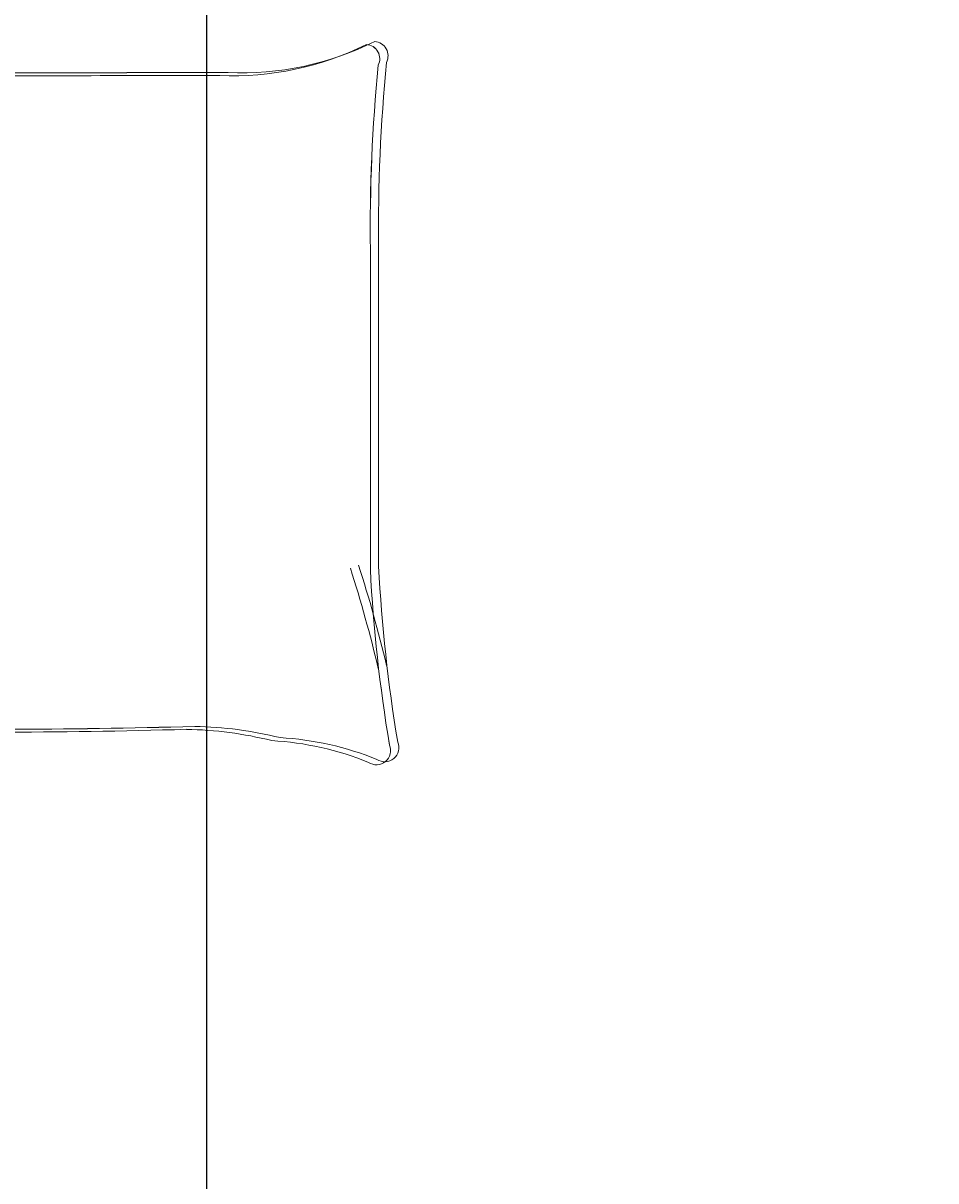
# Model space of a CAD drawing. Units: inches. Extents: x 1601 to 2297, y 1496 to 2631.
# Tile 42 of 57: x 1750 to 1820, y 2391 to 2480. Entities that reach past the tile are written whole.
import ezdxf

# ---------------------------------------------------------------- set-up
doc = ezdxf.new("R2010")
doc.units = ezdxf.units.IN
doc.layers.add('A-ANNO-DIMS', color=2, linetype='Continuous', lineweight=18)
doc.layers.add('A-FURN', color=8, linetype='Continuous', lineweight=18)
doc.styles.get("Standard").update_dxf_attribs({"font": 'arial.ttf'})
doc.dimstyles.get("Standard").update_dxf_attribs({"dimtxt": 0.18, "dimasz": 0.18, "dimexe": 0.18, "dimexo": 0.0625, "dimgap": 0.09, "dimtad": 0, "dimtih": 1, "dimtoh": 1, "dimdec": 4, "dimzin": 0, "dimdsep": 46, "dimtxsty": 'Standard', "dimcen": 0.09, "dimadec": 0, "dimazin": 0, "dimtfac": 1, "dimtdec": 4, "dimtofl": 0, "dimtmove": 0, "dimatfit": 3, "dimfxl": 1, "dimtolj": 1, "dimtzin": 0, "dimarcsym": 0})

# ---------------------------------------------------------------- blocks, each defined once
blk = doc.blocks.new('BED-DOUBLE')
for p, q in [((27.746, 52.867), (24.495, 49.162)), ((27.746, 52.867), (24.495, 49.162)), ((27.746, 52.867), (24.495, 49.162)), ((27.746, 52.867), (24.495, 49.162)), ((28.385, 53.096), (25.135, 49.39)), ((28.385, 53.096), (25.135, 49.39)), ((28.385, 53.096), (25.135, 49.39)), ((28.385, 53.096), (25.135, 49.39)), ((29.49, 52.947), (27.746, 52.867, 3.871)), ((29.49, 52.947), (27.746, 52.867, 3.871)), ((29.49, 52.947), (27.746, 52.867, 3.871)), ((29.49, 52.947), (27.746, 52.867, 3.871)), ((28.365, 51.33), (27.746, 52.867)), ((28.365, 51.33), (27.746, 52.867)), ((28.365, 51.33), (27.746, 52.867)), ((28.365, 51.33), (27.746, 52.867)), ((30.13, 53.175), (28.385, 53.096, 3.871)), ((30.13, 53.175), (28.385, 53.096, 3.871)), ((30.13, 53.175), (28.385, 53.096, 3.871)), ((30.13, 53.175), (28.385, 53.096, 3.871)), ((29.004, 51.559), (28.385, 53.096)), ((29.004, 51.558), (28.385, 53.096)), ((29.004, 51.559), (28.385, 53.096)), ((29.004, 51.558), (28.385, 53.096)), ((0, 51.494), (0.639, 51.493)), ((0, 3.475), (0, 51.494)), ((0, 51.494), (0.639, 51.493)), ((0, 3.475), (0, 51.494)), ((0, 51.265), (26.61, 51.265)), ((0, 51.265), (26.61, 51.265)), ((0, 51.265), (26.61, 51.265)), ((0, 51.265), (26.61, 51.265)), ((0.639, 51.494), (27.249, 51.494)), ((0.639, 51.494), (27.249, 51.494)), ((0.639, 51.493), (27.249, 51.493)), ((0.639, 51.493), (27.249, 51.493)), ((1.533, 3.475), (1.533, 51.265)), ((1.533, 3.475), (1.533, 51.265)), ((1.533, 3.475), (1.533, 51.265)), ((1.533, 3.475), (1.533, 51.265)), ((2.173, 3.703), (2.173, 51.494)), ((2.173, 3.703), (2.173, 51.494)), ((2.173, 3.703), (2.173, 51.493)), ((2.173, 3.703), (2.173, 51.493)), ((17.212, 50.926), (14.073, 50.151)), ((17.212, 50.926), (14.073, 50.151)), ((17.212, 50.926), (14.073, 50.151)), ((17.212, 50.926), (14.073, 50.151)), ((16.808, 45.795), (17.212, 50.926)), ((16.808, 45.794), (17.212, 50.926)), ((16.808, 45.795), (17.212, 50.926)), ((16.808, 45.794), (17.212, 50.926)), ((28.055, 48.233), (28.365, 51.33)), ((28.055, 48.233), (28.365, 51.33)), ((28.055, 48.233), (28.365, 51.33)), ((28.055, 48.233), (28.365, 51.33)), ((28.695, 48.461), (29.004, 51.559)), ((28.695, 48.461), (29.004, 51.559)), ((28.695, 48.461), (29.004, 51.558)), ((28.695, 48.461), (29.004, 51.558)), ((2.557, 50.112), (2.46, 44.709)), ((2.557, 50.112), (2.46, 44.709)), ((2.557, 50.111), (2.46, 44.709)), ((2.557, 50.111), (2.46, 44.709)), ((2.557, 50.112), (5.768, 49.733)), ((2.557, 50.112), (5.768, 49.733)), ((2.557, 50.111), (5.768, 49.733)), ((2.557, 50.111), (5.768, 49.733)), ((3.196, 50.34), (3.099, 44.938)), ((3.196, 50.34), (3.099, 44.938)), ((3.196, 50.34), (3.099, 44.938)), ((3.196, 50.34), (3.099, 44.938)), ((3.196, 50.34), (6.407, 49.961)), ((3.196, 50.34), (6.407, 49.961)), ((3.196, 50.34), (6.407, 49.961)), ((3.196, 50.34), (6.407, 49.961)), ((5.768, 49.733), (8.338, 50.328)), ((5.768, 49.733), (8.338, 50.328)), ((5.768, 49.733), (8.338, 50.328)), ((5.768, 49.733), (8.338, 50.328)), ((6.407, 49.961), (8.977, 50.557)), ((6.407, 49.961), (8.977, 50.557)), ((6.407, 49.961), (8.977, 50.556)), ((6.407, 49.961), (8.977, 50.556)), ((11.829, 50.112), (8.257, 49.309)), ((11.829, 50.112), (8.257, 49.309)), ((11.829, 50.112), (8.257, 49.309)), ((11.829, 50.112), (8.257, 49.309)), ((8.338, 50.328), (9.384, 49.814)), ((8.338, 50.328), (9.384, 49.814)), ((8.338, 50.328), (9.384, 49.814)), ((8.338, 50.328), (9.384, 49.814)), ((12.468, 50.34), (8.896, 49.538)), ((12.468, 50.34), (8.896, 49.537)), ((12.468, 50.34), (8.896, 49.538)), ((12.468, 50.34), (8.896, 49.537)), ((8.977, 50.557), (10.024, 50.043)), ((8.977, 50.557), (10.024, 50.043)), ((8.977, 50.556), (10.024, 50.042)), ((8.977, 50.556), (10.024, 50.042)), ((13.434, 49.923), (11.829, 50.112)), ((13.434, 49.922), (11.829, 50.112)), ((13.434, 49.923), (11.829, 50.112)), ((13.434, 49.922), (11.829, 50.112)), ((14.073, 50.151), (12.468, 50.34)), ((14.073, 50.151), (12.468, 50.34)), ((14.073, 50.151), (12.468, 50.34)), ((14.073, 50.151), (12.468, 50.34)), ((16.573, 50.698), (13.434, 49.923)), ((16.573, 50.698), (13.434, 49.922)), ((16.573, 50.698), (13.434, 49.923)), ((16.573, 50.698), (13.434, 49.922)), ((16.169, 45.566), (16.573, 50.698)), ((16.169, 45.566), (16.573, 50.698)), ((16.169, 45.566), (16.573, 50.698)), ((16.169, 45.566), (16.573, 50.698)), ((8.257, 49.309), (5.578, 48.128)), ((8.257, 49.309), (5.578, 48.128)), ((8.257, 49.309), (5.578, 48.128)), ((8.257, 49.309), (5.578, 48.128)), ((8.896, 49.538), (6.218, 48.356)), ((8.896, 49.538), (6.218, 48.356)), ((8.896, 49.537), (6.218, 48.356)), ((8.896, 49.537), (6.218, 48.356)), ((24.495, 49.162), (22.329, 46.219)), ((24.495, 49.162), (22.329, 46.219)), ((24.495, 49.162), (22.329, 46.219)), ((24.495, 49.162), (22.329, 46.219)), ((25.135, 49.39), (22.968, 46.448)), ((25.135, 49.39), (22.968, 46.448)), ((25.135, 49.39), (22.968, 46.448)), ((25.135, 49.39), (22.968, 46.448)), ((28.365, 44.361), (28.055, 48.233)), ((28.365, 44.361), (28.055, 48.233)), ((28.365, 44.361), (28.055, 48.233)), ((28.365, 44.361), (28.055, 48.233)), ((29.004, 44.589), (28.695, 48.461)), ((29.004, 44.589), (28.695, 48.461)), ((29.004, 44.589), (28.695, 48.461)), ((29.004, 44.589), (28.695, 48.461)), ((22.968, 46.448), (20.956, 40.872)), ((22.968, 46.448), (20.956, 40.872)), ((22.968, 46.448), (20.956, 40.872)), ((22.968, 46.448), (20.956, 40.872)), ((2.46, 44.709), (2.542, 45.712)), ((2.46, 44.709), (2.542, 45.712)), ((2.46, 44.709), (2.542, 45.712)), ((2.46, 44.709), (2.542, 45.712)), ((2.542, 45.712), (3.069, 41.914)), ((2.542, 45.712), (3.069, 41.914)), ((2.542, 45.712), (3.069, 41.914)), ((2.542, 45.712), (3.069, 41.914)), ((3.099, 44.938), (3.181, 45.941)), ((3.099, 44.938), (3.181, 45.941)), ((3.099, 44.938), (3.181, 45.94)), ((3.099, 44.938), (3.181, 45.94)), ((3.181, 45.941), (3.709, 42.143)), ((3.181, 45.941), (3.709, 42.143)), ((3.181, 45.94), (3.709, 42.142)), ((3.181, 45.94), (3.709, 42.142)), ((16.726, 43.606), (16.169, 45.566)), ((16.726, 43.606), (16.169, 45.566)), ((16.726, 43.606), (16.169, 45.566)), ((16.726, 43.606), (16.169, 45.566)), ((17.365, 43.834), (16.808, 45.795)), ((17.365, 43.834), (16.808, 45.795)), ((17.365, 43.834), (16.808, 45.794)), ((17.365, 43.834), (16.808, 45.794)), ((22.329, 46.219), (20.316, 40.644)), ((22.329, 46.219), (20.316, 40.644)), ((22.329, 46.219), (20.317, 40.644)), ((22.329, 46.219), (20.317, 40.644)), ((16.934, 36.824), (17.365, 43.834)), ((16.934, 36.824), (17.365, 43.834)), ((16.934, 36.824), (17.365, 43.834)), ((16.934, 36.824), (17.365, 43.834)), ((28.829, 40.954), (28.365, 44.361)), ((28.829, 40.953), (28.365, 44.361)), ((28.829, 40.954), (28.365, 44.361)), ((28.829, 40.953), (28.365, 44.361)), ((29.468, 41.182), (29.004, 44.589)), ((29.469, 41.182), (29.004, 44.589)), ((29.468, 41.182), (29.004, 44.589)), ((29.469, 41.182), (29.004, 44.589)), ((16.295, 36.596), (16.726, 43.606)), ((16.295, 36.596), (16.726, 43.606)), ((16.295, 36.596), (16.726, 43.606)), ((16.295, 36.596), (16.726, 43.606)), ((3.709, 42.143), (5.061, 36.723)), ((3.709, 42.143), (5.061, 36.723)), ((3.709, 42.142), (5.061, 36.723)), ((3.709, 42.142), (5.061, 36.723)), ((3.069, 41.914), (4.422, 36.495)), ((3.069, 41.914), (4.422, 36.495)), ((3.069, 41.914), (4.422, 36.495)), ((3.069, 41.914), (4.422, 36.495)), ((30.397, 39.169), (29.468, 41.182)), ((30.397, 39.169), (29.468, 41.182)), ((30.397, 39.168), (29.469, 41.182)), ((30.397, 39.168), (29.469, 41.182)), ((20.316, 40.644), (17.383, 32.306)), ((20.317, 40.644), (17.383, 32.306)), ((20.316, 40.644), (17.383, 32.306)), ((20.317, 40.644), (17.383, 32.306)), ((20.956, 40.872), (18.022, 32.534)), ((20.956, 40.872), (18.022, 32.534)), ((20.956, 40.872), (18.022, 32.534)), ((20.956, 40.872), (18.022, 32.534)), ((29.758, 38.94), (28.829, 40.954)), ((29.758, 38.94), (28.829, 40.954)), ((29.758, 38.94), (28.829, 40.953)), ((29.758, 38.94), (28.829, 40.953)), ((4.313, 39.428), (3.717, 37.363)), ((4.313, 39.428), (3.717, 37.363)), ((4.313, 39.428), (3.718, 37.363)), ((4.313, 39.428), (3.718, 37.363)), ((79.245, 15.063), (79.245, 39.677)), ((79.245, 15.063), (79.245, 39.677)), ((79.245, 15.063), (79.245, 39.677)), ((79.245, 15.063), (79.245, 39.677)), ((79.884, 15.292), (79.884, 39.905)), ((79.884, 15.291), (79.884, 39.905)), ((79.884, 15.292), (79.884, 39.905)), ((79.884, 15.291), (79.884, 39.905)), ((3.673, 39.2), (3.078, 37.135)), ((3.673, 39.2), (3.078, 37.135)), ((3.673, 39.2), (3.078, 37.135)), ((3.673, 39.2), (3.078, 37.135)), ((30.377, 36.462), (29.758, 38.94)), ((30.377, 36.462), (29.758, 38.94)), ((30.377, 36.462), (29.758, 38.94)), ((30.377, 36.462), (29.758, 38.94)), ((31.016, 36.691), (30.397, 39.169)), ((31.016, 36.691), (30.397, 39.169)), ((31.016, 36.691), (30.397, 39.168)), ((31.016, 36.691), (30.397, 39.168)), ((3.078, 37.135), (2.537, 34.204)), ((3.078, 37.135), (2.537, 34.204)), ((3.078, 37.135), (2.537, 34.204)), ((3.078, 37.135), (2.537, 34.204)), ((3.717, 37.363), (3.176, 34.433)), ((3.718, 37.363), (3.176, 34.433)), ((3.717, 37.363), (3.176, 34.433)), ((3.718, 37.363), (3.176, 34.433)), ((15.628, 32.564), (16.295, 36.596)), ((15.628, 32.564), (16.295, 36.596)), ((15.628, 32.564), (16.295, 36.596)), ((15.628, 32.564), (16.295, 36.596)), ((16.268, 32.792), (16.934, 36.824)), ((16.268, 32.792), (16.934, 36.824)), ((16.268, 32.792), (16.934, 36.824)), ((16.268, 32.792), (16.934, 36.824)), ((29.004, 36.381), (31.016, 36.691)), ((29.004, 36.381), (31.016, 36.691)), ((29.004, 36.381), (31.016, 36.691)), ((29.004, 36.381), (31.016, 36.691)), ((23.876, 34.449), (28.365, 36.153)), ((23.876, 34.449), (28.365, 36.153)), ((23.876, 34.449), (28.365, 36.152)), ((23.876, 34.449), (28.365, 36.152)), ((24.516, 34.677), (29.004, 36.381)), ((24.516, 34.677), (29.004, 36.381)), ((24.516, 34.677), (29.004, 36.381)), ((24.516, 34.677), (29.004, 36.381)), ((28.365, 36.153), (30.377, 36.462)), ((28.365, 36.152), (30.377, 36.462)), ((28.365, 36.153), (30.377, 36.462)), ((28.365, 36.152), (30.377, 36.462)), ((2.537, 34.204), (2.557, 33.883)), ((2.537, 34.204), (2.557, 33.883)), ((2.537, 34.204), (2.557, 33.883)), ((2.537, 34.204), (2.557, 33.883)), ((3.176, 34.433), (3.196, 34.112)), ((3.176, 34.433), (3.196, 34.112)), ((3.176, 34.433), (3.196, 34.112)), ((3.176, 34.433), (3.196, 34.112)), ((3.196, 34.112), (3.618, 29.684)), ((3.196, 34.112), (3.618, 29.684)), ((3.196, 34.112), (3.618, 29.684)), ((3.196, 34.112), (3.618, 29.684)), ((17.379, 30.978), (16.094, 34.049)), ((17.379, 30.978), (16.094, 34.049)), ((17.379, 30.978), (16.094, 34.049)), ((17.379, 30.978), (16.094, 34.049)), ((17.383, 30.259), (23.876, 34.449)), ((17.383, 30.259), (23.876, 34.449)), ((17.383, 30.259), (23.876, 34.449)), ((17.383, 30.259), (23.876, 34.449)), ((18.022, 30.487), (24.516, 34.677)), ((18.022, 30.487), (24.516, 34.677)), ((18.022, 30.487), (24.516, 34.677)), ((18.022, 30.487), (24.516, 34.677)), ((2.557, 33.883), (2.979, 29.456)), ((2.557, 33.883), (2.979, 29.455)), ((2.557, 33.883), (2.979, 29.456)), ((2.557, 33.883), (2.979, 29.455)), ((16.739, 30.75), (15.454, 33.821)), ((16.739, 30.75), (15.454, 33.821)), ((16.739, 30.75), (15.454, 33.82)), ((16.739, 30.75), (15.454, 33.82)), ((16.893, 28.297), (16.739, 30.75)), ((16.893, 28.297), (16.739, 30.75)), ((16.893, 28.297), (16.739, 30.75)), ((16.893, 28.297), (16.739, 30.75)), ((17.532, 28.526), (17.379, 30.978)), ((17.532, 28.525), (17.379, 30.978)), ((17.532, 28.526), (17.379, 30.978)), ((17.532, 28.525), (17.379, 30.978)), ((2.979, 29.456), (2.492, 27.977)), ((2.979, 29.456), (2.492, 27.977)), ((2.979, 29.455), (2.492, 27.976)), ((2.979, 29.455), (2.492, 27.976)), ((3.618, 29.684), (3.131, 28.205)), ((3.618, 29.684), (3.131, 28.205)), ((3.618, 29.684), (3.131, 28.205)), ((3.618, 29.684), (3.131, 28.205)), ((2.492, 27.977), (7.867, 27.733)), ((2.492, 27.977), (7.867, 27.733)), ((2.492, 27.976), (7.867, 27.733)), ((2.492, 27.976), (7.867, 27.733)), ((3.131, 28.205), (8.506, 27.962)), ((3.131, 28.205), (8.506, 27.961)), ((3.131, 28.205), (8.506, 27.962)), ((3.131, 28.205), (8.506, 27.961)), ((7.867, 27.733), (11.078, 27.355)), ((7.867, 27.733), (11.078, 27.354)), ((7.867, 27.733), (11.078, 27.355)), ((7.867, 27.733), (11.078, 27.354)), ((8.506, 27.962), (11.717, 27.583)), ((8.506, 27.962), (11.717, 27.583)), ((8.506, 27.961), (11.717, 27.583)), ((8.506, 27.961), (11.717, 27.583)), ((11.717, 27.583), (13.016, 27.664)), ((11.717, 27.583), (13.016, 27.664)), ((11.717, 27.583), (13.016, 27.664)), ((11.717, 27.583), (13.016, 27.664)), ((12.377, 27.436), (14.216, 28.13)), ((12.377, 27.436), (14.217, 28.13)), ((12.377, 27.436), (14.216, 28.13)), ((12.377, 27.436), (14.217, 28.13)), ((13.016, 27.664), (14.856, 28.359)), ((13.016, 27.664), (14.856, 28.359)), ((13.016, 27.664), (14.856, 28.358)), ((13.016, 27.664), (14.856, 28.358)), ((14.216, 28.13), (16.893, 28.297)), ((14.216, 28.13), (16.893, 28.297)), ((14.217, 28.13), (16.893, 28.297)), ((14.217, 28.13), (16.893, 28.297)), ((14.856, 28.359), (17.532, 28.526)), ((14.856, 28.359), (17.532, 28.526)), ((14.856, 28.358), (17.532, 28.525)), ((14.856, 28.358), (17.532, 28.525)), ((2.509, 26.211), (7.859, 26.789)), ((2.509, 26.21), (7.859, 26.789)), ((2.509, 26.211), (7.859, 26.789)), ((2.509, 26.21), (7.859, 26.789)), ((7.22, 26.561), (10.401, 27.139)), ((7.22, 26.56), (10.401, 27.139)), ((7.22, 26.561), (10.401, 27.139)), ((7.22, 26.56), (10.401, 27.139)), ((7.859, 26.789), (11.04, 27.367)), ((7.859, 26.789), (11.04, 27.367)), ((7.859, 26.789), (11.04, 27.367)), ((7.859, 26.789), (11.04, 27.367)), ((10.401, 27.139), (11.702, 27.139)), ((10.401, 27.139), (11.702, 27.139)), ((10.401, 27.139), (11.702, 27.139)), ((10.401, 27.139), (11.702, 27.139)), ((11.04, 27.367), (12.341, 27.367)), ((11.04, 27.367), (12.341, 27.367)), ((11.04, 27.367), (12.341, 27.367)), ((11.04, 27.367), (12.341, 27.367)), ((11.078, 27.355), (12.377, 27.436)), ((11.078, 27.354), (12.377, 27.436)), ((11.078, 27.355), (12.377, 27.436)), ((11.078, 27.354), (12.377, 27.436)), ((11.702, 27.139), (13.582, 26.561)), ((11.702, 27.139), (13.582, 26.56)), ((11.702, 27.139), (13.582, 26.561)), ((11.702, 27.139), (13.582, 26.56)), ((12.341, 27.367), (14.221, 26.789)), ((12.341, 27.367), (14.221, 26.789)), ((12.341, 27.367), (14.221, 26.789)), ((12.341, 27.367), (14.221, 26.789)), ((14.221, 26.789), (16.902, 26.789)), ((14.221, 26.789), (16.902, 26.789)), ((14.221, 26.789), (16.902, 26.789)), ((14.221, 26.789), (16.902, 26.789)), ((16.902, 26.789), (16.902, 24.332)), ((16.902, 26.789), (16.902, 24.331)), ((16.902, 26.789), (16.902, 24.332)), ((16.902, 26.789), (16.902, 24.331)), ((1.87, 25.982), (7.22, 26.561)), ((1.87, 25.982), (7.22, 26.561)), ((1.87, 25.982), (7.22, 26.56)), ((1.87, 25.982), (7.22, 26.56)), ((2.448, 24.537), (1.87, 25.982)), ((2.448, 24.537), (1.87, 25.982)), ((2.448, 24.537), (1.87, 25.982)), ((2.448, 24.537), (1.87, 25.982)), ((3.088, 24.765), (2.509, 26.211)), ((3.088, 24.765), (2.509, 26.211)), ((3.088, 24.765), (2.509, 26.21)), ((3.088, 24.765), (2.509, 26.21)), ((13.582, 26.561), (16.263, 26.561)), ((13.582, 26.561), (16.263, 26.561)), ((13.582, 26.56), (16.263, 26.56)), ((13.582, 26.56), (16.263, 26.56)), ((16.263, 26.561), (16.263, 24.103)), ((16.263, 26.561), (16.263, 24.103)), ((16.263, 26.56), (16.263, 24.103)), ((16.263, 26.56), (16.263, 24.103)), ((2.304, 20.091), (2.448, 24.537)), ((2.304, 20.091), (2.448, 24.537)), ((2.304, 20.091), (2.448, 24.537)), ((2.304, 20.091), (2.448, 24.537)), ((2.943, 20.32), (3.088, 24.765)), ((2.943, 20.319), (3.088, 24.765)), ((2.943, 20.32), (3.088, 24.765)), ((2.943, 20.319), (3.088, 24.765)), ((16.263, 24.103), (15.172, 20.959)), ((16.263, 24.103), (15.172, 20.958)), ((16.263, 24.103), (15.172, 20.959)), ((16.263, 24.103), (15.172, 20.958)), ((16.902, 24.332), (15.811, 21.187)), ((16.902, 24.332), (15.811, 21.187)), ((16.902, 24.331), (15.811, 21.187)), ((16.902, 24.331), (15.811, 21.187)), ((16.169, 19.384), (16.573, 24.516)), ((16.169, 19.384), (16.573, 24.516)), ((16.169, 19.383), (16.573, 24.515)), ((16.169, 19.383), (16.573, 24.515)), ((16.808, 19.612), (17.212, 24.744)), ((16.808, 19.612), (17.212, 24.744)), ((16.808, 19.612), (17.212, 24.744)), ((16.808, 19.612), (17.212, 24.744)), ((2.304, 19.77), (2.304, 20.091)), ((2.304, 19.769), (2.304, 20.091)), ((2.304, 19.77), (2.304, 20.091)), ((2.304, 19.769), (2.304, 20.091)), ((3.027, 16.878), (2.304, 19.77)), ((3.027, 16.878), (2.304, 19.77)), ((3.027, 16.878), (2.304, 19.769)), ((3.027, 16.878), (2.304, 19.769)), ((2.943, 19.998), (2.943, 20.32)), ((2.943, 19.998), (2.943, 20.32)), ((2.943, 19.998), (2.943, 20.319)), ((2.943, 19.998), (2.943, 20.319)), ((3.666, 17.107), (2.943, 19.998)), ((3.666, 17.107), (2.943, 19.998)), ((3.666, 17.107), (2.943, 19.998)), ((3.666, 17.107), (2.943, 19.998)), ((16.726, 17.423), (16.169, 19.384)), ((16.726, 17.423), (16.169, 19.384)), ((16.726, 17.423), (16.169, 19.383)), ((16.726, 17.423), (16.169, 19.383)), ((17.365, 17.652), (16.808, 19.612)), ((17.365, 17.651), (16.808, 19.612)), ((17.365, 17.652), (16.808, 19.612)), ((17.365, 17.651), (16.808, 19.612)), ((3.316, 12.108), (4.328, 17.601)), ((3.316, 12.108), (4.328, 17.601)), ((3.316, 12.108), (4.328, 17.601)), ((3.316, 12.108), (4.328, 17.601)), ((4.389, 15.083), (3.666, 17.107)), ((4.389, 15.083), (3.666, 17.107)), ((4.389, 15.083), (3.666, 17.107)), ((4.389, 15.083), (3.666, 17.107)), ((3.955, 12.336), (4.967, 17.83)), ((3.955, 12.336), (4.967, 17.83)), ((3.955, 12.336), (4.967, 17.829)), ((3.955, 12.336), (4.967, 17.829)), ((16.295, 10.413), (16.726, 17.423)), ((16.295, 10.413), (16.726, 17.423)), ((16.295, 10.413), (16.726, 17.423)), ((16.295, 10.413), (16.726, 17.423)), ((16.934, 10.642), (17.365, 17.652)), ((16.934, 10.642), (17.365, 17.652)), ((16.934, 10.642), (17.365, 17.651)), ((16.934, 10.642), (17.365, 17.651)), ((3.75, 14.855), (3.027, 16.878)), ((3.75, 14.854), (3.027, 16.878)), ((3.75, 14.855), (3.027, 16.878)), ((3.75, 14.854), (3.027, 16.878)), ((3.027, 8.285), (3.316, 12.108)), ((3.027, 8.284), (3.316, 12.108)), ((3.027, 8.285), (3.316, 12.108)), ((3.027, 8.284), (3.316, 12.108)), ((3.666, 8.513), (3.955, 12.336)), ((3.666, 8.513), (3.955, 12.336)), ((3.666, 8.513), (3.955, 12.336)), ((3.666, 8.513), (3.955, 12.336)), ((15.628, 6.382), (16.295, 10.413)), ((15.628, 6.381), (16.295, 10.413)), ((15.628, 6.382), (16.295, 10.413)), ((15.628, 6.381), (16.295, 10.413)), ((16.268, 6.61), (16.934, 10.642)), ((16.268, 6.61), (16.934, 10.642)), ((16.268, 6.61), (16.934, 10.642)), ((16.268, 6.61), (16.934, 10.642)), ((16.295, 10.413), (16.618, 9.28)), ((16.295, 10.413), (16.618, 9.28)), ((16.295, 10.413), (16.618, 9.28)), ((16.295, 10.413), (16.618, 9.28)), ((16.934, 10.642), (17.257, 9.509)), ((16.934, 10.642), (17.257, 9.508)), ((16.934, 10.642), (17.257, 9.509)), ((16.934, 10.642), (17.257, 9.508)), ((16.618, 9.28), (17.341, 4.184)), ((16.618, 9.28), (17.341, 4.183)), ((16.618, 9.28), (17.341, 4.184)), ((16.618, 9.28), (17.341, 4.183)), ((17.257, 9.509), (17.98, 4.412)), ((17.257, 9.509), (17.98, 4.412)), ((17.257, 9.508), (17.98, 4.412)), ((17.257, 9.508), (17.98, 4.412)), ((3.009, 8.179), (3.027, 8.285)), ((3.009, 8.179), (3.027, 8.285)), ((3.009, 8.179), (3.027, 8.284)), ((3.009, 8.179), (3.027, 8.284)), ((3.338, 3.898), (3.009, 8.179)), ((3.338, 3.898), (3.009, 8.179)), ((3.338, 3.898), (3.009, 8.179)), ((3.338, 3.898), (3.009, 8.179)), ((3.648, 8.408), (3.666, 8.513)), ((3.648, 8.407), (3.666, 8.513)), ((3.648, 8.408), (3.666, 8.513)), ((3.648, 8.407), (3.666, 8.513)), ((3.977, 4.127), (3.648, 8.408)), ((3.977, 4.127), (3.648, 8.408)), ((3.977, 4.127), (3.648, 8.407)), ((3.977, 4.127), (3.648, 8.407)), ((9.594, 5.279), (6.847, 6.291)), ((9.594, 5.279), (6.847, 6.291)), ((9.594, 5.279), (6.847, 6.291)), ((9.594, 5.279), (6.847, 6.291)), ((8.955, 5.051), (6.208, 6.063)), ((8.955, 5.051), (6.208, 6.063)), ((8.955, 5.051), (6.208, 6.063)), ((8.955, 5.051), (6.208, 6.063)), ((3.316, 3.894), (6.497, 4.473)), ((3.316, 3.894), (6.497, 4.473)), ((3.316, 3.894), (6.497, 4.472)), ((3.316, 3.894), (6.497, 4.472)), ((3.955, 4.123), (7.136, 4.701)), ((3.955, 4.123), (7.136, 4.701)), ((3.955, 4.123), (7.136, 4.701)), ((3.955, 4.123), (7.136, 4.701)), ((6.497, 4.473), (9.099, 4.039)), ((6.497, 4.473), (9.099, 4.039)), ((6.497, 4.472), (9.099, 4.039)), ((6.497, 4.472), (9.099, 4.039)), ((7.136, 4.701), (9.739, 4.267)), ((7.136, 4.701), (9.739, 4.267)), ((7.136, 4.701), (9.739, 4.267)), ((7.136, 4.701), (9.739, 4.267)), ((12.57, 4.473), (8.955, 5.051)), ((12.57, 4.472), (8.955, 5.051)), ((12.57, 4.473), (8.955, 5.051)), ((12.57, 4.472), (8.955, 5.051)), ((9.099, 4.039), (10.112, 4.617)), ((9.099, 4.039), (10.112, 4.617)), ((9.099, 4.039), (10.112, 4.617)), ((9.099, 4.039), (10.112, 4.617)), ((13.209, 4.701), (9.594, 5.279)), ((13.209, 4.701), (9.594, 5.279)), ((13.209, 4.701), (9.594, 5.279)), ((13.209, 4.701), (9.594, 5.279)), ((9.739, 4.267), (10.751, 4.846)), ((9.739, 4.267), (10.751, 4.846)), ((9.739, 4.267), (10.751, 4.845)), ((9.739, 4.267), (10.751, 4.845)), ((14.16, 4.762), (12.57, 4.473)), ((14.16, 4.762), (12.57, 4.472)), ((14.16, 4.762), (12.57, 4.473)), ((14.16, 4.762), (12.57, 4.472)), ((14.799, 4.99), (13.209, 4.701)), ((14.799, 4.99), (13.209, 4.701)), ((14.799, 4.99), (13.209, 4.701)), ((14.799, 4.99), (13.209, 4.701)), ((17.341, 4.184), (14.16, 4.762)), ((17.341, 4.183), (14.16, 4.762)), ((17.341, 4.184), (14.16, 4.762)), ((17.341, 4.183), (14.16, 4.762)), ((17.98, 4.412), (14.799, 4.99)), ((17.98, 4.412), (14.799, 4.99)), ((17.98, 4.412), (14.799, 4.99)), ((17.98, 4.412), (14.799, 4.99)), ((18.75, 3.703), (0.639, 3.703)), ((18.75, 3.703), (0.639, 3.703)), ((18.75, 3.703), (0.639, 3.703)), ((18.75, 3.703), (0.639, 3.703)), ((18.11, 3.475), (0, 3.475)), ((18.11, 3.475), (0, 3.475)), ((18.11, 3.475), (0, 3.475)), ((18.11, 3.475), (0, 3.475))]:
    blk.add_line(p, q)
for centre, radius, start, end in [((68.666, 76.157), 23.065, 267.47136, 296.46809), ((68.666, 76.157), 23.065, 267.47136, 296.46809), ((68.666, 76.157), 23.065, 267.47136, 296.46809), ((68.666, 76.157), 23.065, 267.47136, 296.46809), ((69.306, 76.385), 23.065, 267.47136, 296.46809), ((69.306, 76.385), 23.065, 267.47136, 296.46809), ((69.306, 76.385), 23.065, 267.47136, 296.46809), ((69.306, 76.385), 23.065, 267.47136, 296.46809), ((78.87, 54.41), 1.102, 332.65876, 86.02002), ((78.87, 54.409), 1.102, 332.65876, 86.02002), ((78.87, 54.41), 1.102, 332.65876, 86.02002), ((78.87, 54.409), 1.102, 332.65876, 86.02002), ((79.509, 54.638), 1.102, 332.65876, 86.02002), ((79.509, 54.638), 1.102, 332.65876, 86.02002), ((79.509, 54.638), 1.102, 332.65876, 86.02002), ((79.509, 54.638), 1.102, 332.65876, 86.02002), ((212.276, 41.152), 133.04, 174.4998, 180.63509), ((212.277, 41.151), 133.04, 174.4998, 180.63509), ((212.276, 41.152), 133.04, 174.4998, 180.63509), ((212.277, 41.151), 133.04, 174.4998, 180.63509), ((212.916, 41.38), 133.04, 174.4998, 180.63509), ((212.916, 41.38), 133.04, 174.4998, 180.63509), ((212.916, 41.38), 133.04, 174.4998, 180.63509), ((212.916, 41.38), 133.04, 174.4998, 180.63509), ((-6.656, 51.327), 36.183, 349.87628, 2.56571), ((-6.656, 51.327), 36.183, 349.87628, 2.56571), ((-6.656, 51.327), 36.183, 349.87628, 2.56571), ((-6.656, 51.327), 36.183, 349.87628, 2.56571), ((36.315, 182.266), 129.499, 266.97912, 273.83645), ((36.315, 182.265), 129.499, 266.97912, 273.83645), ((36.315, 182.266), 129.499, 266.97912, 273.83645), ((36.315, 182.265), 129.499, 266.97912, 273.83645), ((-6.017, 51.555), 36.183, 349.87628, 2.56571), ((-6.017, 51.555), 36.183, 349.87628, 2.56571), ((-6.017, 51.555), 36.183, 349.87628, 2.56571), ((-6.017, 51.555), 36.183, 349.87628, 2.56571), ((36.954, 182.494), 129.499, 266.97912, 273.83645), ((36.954, 182.494), 129.499, 266.97912, 273.83645), ((36.954, 182.494), 129.499, 266.97912, 273.83645), ((36.954, 182.494), 129.499, 266.97912, 273.83645), ((67.821, -4508.744), 4561.858, 90.002168, 90.286887), ((67.821, -4508.744), 4561.858, 90.002168, 90.286887), ((67.821, -4508.744), 4561.858, 90.002168, 90.286887), ((67.821, -4508.744), 4561.858, 90.002168, 90.286887), ((68.461, -4508.515), 4561.858, 90.002168, 90.286887), ((68.461, -4508.515), 4561.858, 90.002168, 90.286887), ((68.461, -4508.516), 4561.858, 90.002168, 90.286887), ((68.461, -4508.516), 4561.858, 90.002168, 90.286887), ((35.066, 43.743), 6.224, 168.6608, 203.73842), ((35.066, 43.743), 6.224, 168.6608, 203.73842), ((35.066, 43.743), 6.224, 168.6608, 203.73842), ((35.066, 43.743), 6.224, 168.6608, 203.73842), ((35.705, 43.972), 6.224, 168.6608, 203.73842), ((35.705, 43.971), 6.224, 168.6608, 203.73842), ((35.705, 43.972), 6.224, 168.6608, 203.73842), ((35.705, 43.971), 6.224, 168.6608, 203.73842), ((1.482, 31.154), 29.654, 10.66171, 19.88058), ((1.482, 31.154), 29.654, 10.66171, 19.88058), ((1.482, 31.153), 29.654, 10.66171, 19.88058), ((1.482, 31.153), 29.654, 10.66171, 19.88058), ((2.121, 31.382), 29.654, 10.66171, 19.88058), ((2.121, 31.382), 29.654, 10.66171, 19.88058), ((2.121, 31.382), 29.654, 10.66171, 19.88058), ((2.121, 31.382), 29.654, 10.66171, 19.88058), ((30.439, 36.636), 0.185, 250.24637, 1.13765), ((30.439, 36.636), 0.185, 250.24637, 1.13765), ((30.439, 36.636), 0.185, 250.24637, 1.13765), ((30.439, 36.636), 0.185, 250.24637, 1.13765), ((31.079, 36.864), 0.185, 250.24637, 1.13765), ((31.079, 36.864), 0.185, 250.24637, 1.13765), ((31.079, 36.864), 0.185, 250.24637, 1.13765), ((31.079, 36.864), 0.185, 250.24637, 1.13765), ((156.316, 17.756), 129.02, 171.78449, 186.90062), ((156.316, 17.755), 129.02, 171.78449, 186.90062), ((156.316, 17.756), 129.02, 171.78449, 186.90062), ((156.316, 17.755), 129.02, 171.78449, 186.90062), ((156.955, 17.984), 129.02, 171.78449, 186.90062), ((156.955, 17.984), 129.02, 171.78449, 186.90062), ((156.955, 17.984), 129.02, 171.78449, 186.90062), ((156.955, 17.984), 129.02, 171.78449, 186.90062), ((182.052, 21.359), 164.969, 176.08655, 186.78213), ((182.052, 21.359), 164.969, 176.08655, 186.78213), ((182.052, 21.358), 164.969, 176.08655, 186.78213), ((182.052, 21.358), 164.969, 176.08655, 186.78213), ((182.692, 21.587), 164.969, 176.08655, 186.78213), ((182.692, 21.587), 164.969, 176.08655, 186.78213), ((182.692, 21.587), 164.969, 176.08655, 186.78213), ((182.692, 21.587), 164.969, 176.08655, 186.78213), ((-23.073, -16.994), 106.459, 13.38322, 17.70533), ((-23.073, -16.994), 106.459, 13.38322, 17.70533), ((-23.073, -16.994), 106.459, 13.38322, 17.70533), ((-23.073, -16.994), 106.459, 13.38322, 17.70533), ((201.476, 21.655), 121.759, 182.99578, 189.40907), ((201.476, 21.655), 121.759, 182.99578, 189.40907), ((201.476, 21.655), 121.759, 182.99578, 189.40907), ((201.476, 21.655), 121.759, 182.99578, 189.40907), ((-23.712, -17.222), 106.459, 13.38322, 17.70533), ((-23.712, -17.222), 106.459, 13.38322, 17.70533), ((-23.712, -17.222), 106.459, 13.38322, 17.70533), ((-23.712, -17.222), 106.459, 13.38322, 17.70533), ((200.837, 21.427), 121.759, 182.99578, 189.40907), ((200.837, 21.426), 121.759, 182.99578, 189.40907), ((200.837, 21.427), 121.759, 182.99578, 189.40907), ((200.837, 21.426), 121.759, 182.99578, 189.40907), ((31.174, -167.308), 170.11, 88.4762, 91.00819), ((31.174, -167.308), 170.11, 88.4762, 91.00819), ((31.174, -167.308), 170.11, 88.4762, 91.00819), ((31.174, -167.308), 170.11, 88.4762, 91.00819), ((31.813, -167.079), 170.11, 88.4762, 91.00819), ((31.813, -167.08), 170.11, 88.4762, 91.00819), ((31.813, -167.079), 170.11, 88.4762, 91.00819), ((31.813, -167.08), 170.11, 88.4762, 91.00819), ((50.614, 484.822), 482.31, 268.22771, 271.71854), ((50.614, 484.822), 482.31, 268.22771, 271.71854), ((50.614, 484.822), 482.31, 268.22771, 271.71854), ((50.614, 484.822), 482.31, 268.22771, 271.71854), ((51.253, 485.051), 482.31, 268.22771, 271.71854), ((51.253, 485.05), 482.31, 268.22771, 271.71854), ((51.253, 485.051), 482.31, 268.22771, 271.71854), ((51.253, 485.05), 482.31, 268.22771, 271.71854), ((64.515, -26.9), 29.634, 76.06484, 88.91125), ((64.515, -26.9), 29.634, 76.06484, 88.91125), ((64.515, -26.9), 29.634, 76.06484, 88.91125), ((64.515, -26.9), 29.634, 76.06484, 88.91125), ((65.154, -26.671), 29.634, 76.06484, 88.91125), ((65.154, -26.672), 29.634, 76.06484, 88.91125), ((65.154, -26.671), 29.634, 76.06484, 88.91125), ((65.154, -26.672), 29.634, 76.06484, 88.91125), ((20.096, 85.162), 83.306, 268.72178, 275.60397), ((20.096, 85.161), 83.306, 268.72178, 275.60397), ((20.096, 85.162), 83.306, 268.72178, 275.60397), ((20.096, 85.161), 83.306, 268.72178, 275.60397), ((20.735, 85.39), 83.306, 268.72178, 275.60397), ((20.735, 85.39), 83.306, 268.72178, 275.60397), ((20.736, 85.39), 83.306, 268.72178, 275.60397), ((20.736, 85.39), 83.306, 268.72178, 275.60397), ((70.276, -21.66), 23.562, 67.97508, 86.652), ((70.276, -21.66), 23.562, 67.97508, 86.652), ((70.276, -21.66), 23.562, 67.97508, 86.652), ((70.276, -21.66), 23.562, 67.97508, 86.652), ((70.915, -21.431), 23.562, 67.97508, 86.652), ((70.915, -21.432), 23.562, 67.97508, 86.652), ((70.915, -21.431), 23.562, 67.97508, 86.652), ((70.915, -21.432), 23.562, 67.97508, 86.652), ((79.718, 1.087), 1.089, 236.17358, 23.47814), ((79.718, 1.087), 1.089, 236.17358, 23.47814), ((79.718, 1.087), 1.089, 236.17358, 23.47814), ((79.718, 1.087), 1.089, 236.17358, 23.47814), ((80.357, 1.316), 1.089, 236.17358, 23.47814), ((80.357, 1.316), 1.089, 236.17358, 23.47814), ((80.357, 1.315), 1.089, 236.17358, 23.47814), ((80.357, 1.315), 1.089, 236.17358, 23.47814)]:
    blk.add_arc(centre, radius, start, end)
blk = doc.blocks.new('*D33')
at = {"layer": 'A-ANNO-DIMS', "color": 0, "lineweight": -2, "transparency": 16777216}
for p, q in [((1764.337, 2136.388), (1764.337, 2581.055)), ((1764.517, 2580.875), (1816.057, 2580.875)), ((1868.157, 2580.875), (1816.617, 2580.875)), ((1868.337, 2136.388), (1868.337, 2581.055))]:
    blk.add_line(p, q, dxfattribs=at)
at = {"layer": 'A-ANNO-DIMS', "color": 0, "transparency": 16777216}
for points in [[(1764.517, 2580.905), (1764.517, 2580.845), (1764.337, 2580.875)], [(1868.157, 2580.905), (1868.157, 2580.845), (1868.337, 2580.875)]]:
    blk.add_solid(points, dxfattribs=at)
at = {"layer": 'Defpoints', "color": 0, "transparency": 16777216}
for p in [(1868.337, 2580.875), (1764.337, 2136.325), (1868.337, 2136.325)]:
    blk.add_point(p, dxfattribs=at)
at = {"layer": 'A-ANNO-DIMS', "color": 0, "transparency": 16777216, "insert": (1816.337, 2580.875), "char_height": 0.18, "attachment_point": 5}
blk.add_mtext('\\A1;104', dxfattribs=at)

msp = doc.modelspace()

# ---------------------------------------------------------------- block references
at = {"layer": 'A-FURN'}
msp.add_blockref('BED-DOUBLE', (1697.682, 2423.048), dxfattribs=at)

# ---------------------------------------------------------------- dimensions: what is measured, and where the dimension line sits
at = {"layer": 'A-ANNO-DIMS'}
dim = msp.add_linear_dim(base=(1868.3371, 2580.8754), p1=(1764.3371, 2136.3254), p2=(1868.3371, 2136.3254), dimstyle='Standard', override={"dimdec": 0, "dimlfac": 1, "dimrnd": 0, "dimzin": 0, "dimdsep": 46, "dimlunit": 2}, dxfattribs=at)
dim.commit()
dim.dimension.update_dxf_attribs({"geometry": '*D33', "text_midpoint": (1816.3371, 2580.8754)})

doc.saveas('drawing.dxf')
